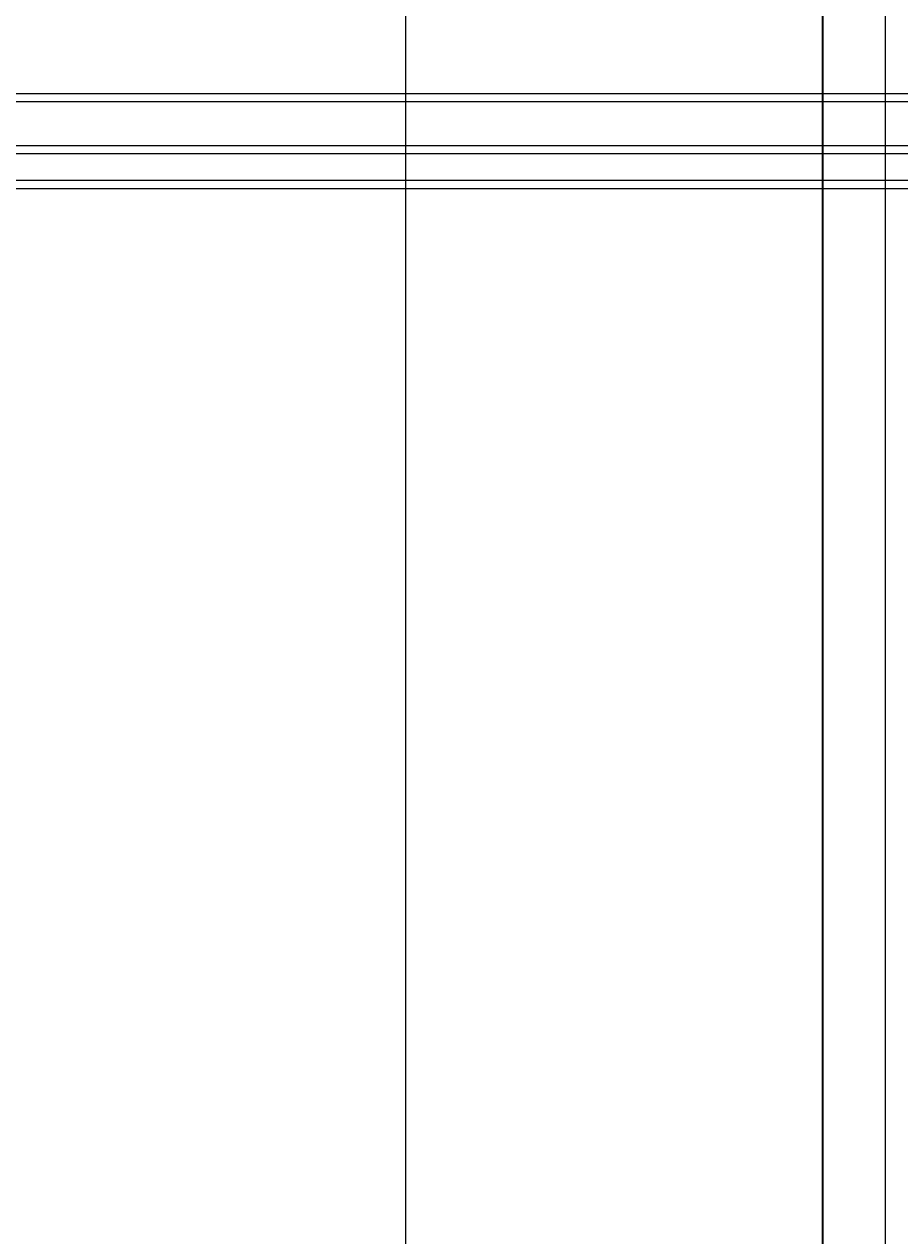
# Model space of a CAD drawing. Units: inches. Extents: x -6 to 289, y -8 to 323.
# Tile 75 of 107: x 248 to 273, y 194 to 229. Entities that reach past the tile are written whole.
import ezdxf

# ---------------------------------------------------------------- set-up
doc = ezdxf.new("R2010")
doc.units = ezdxf.units.IN
doc.header["$MEASUREMENT"] = 0
doc.layers.add('A-ANNO-DIMS', color=2, linetype='Continuous', lineweight=18)
doc.layers.add('A-ELEV', color=7, linetype='Continuous', lineweight=35)
doc.styles.get("Standard").update_dxf_attribs({"font": 'arial.ttf'})
doc.dimstyles.get("Standard").update_dxf_attribs({"dimtxt": 0.18, "dimasz": 0.18, "dimexe": 0.18, "dimexo": 0.0625, "dimgap": 0.09, "dimtad": 0, "dimtih": 1, "dimtoh": 1, "dimdec": 4, "dimzin": 0, "dimdsep": 46, "dimtxsty": 'Standard', "dimcen": 0.09, "dimadec": 0, "dimazin": 0, "dimtfac": 1, "dimtdec": 4, "dimtofl": 0, "dimtmove": 0, "dimatfit": 3, "dimfxl": 1, "dimtolj": 1, "dimtzin": 0, "dimarcsym": 0})

# ---------------------------------------------------------------- blocks, each defined once
blk = doc.blocks.new('*D15')
at = {"layer": 'A-ANNO-DIMS', "color": 0, "lineweight": -2, "transparency": 16777216}
for p, q in [((247.164, 162.411), (247.164, 322.969)), ((271.164, 7.351), (271.164, 322.969)), ((247.344, 322.789), (258.944, 322.789)), ((270.984, 322.789), (259.384, 322.789))]:
    blk.add_line(p, q, dxfattribs=at)
at = {"layer": 'A-ANNO-DIMS', "color": 0, "transparency": 16777216}
for points in [[(247.344, 322.819), (247.344, 322.759), (247.164, 322.789)], [(270.984, 322.819), (270.984, 322.759), (271.164, 322.789)]]:
    blk.add_solid(points, dxfattribs=at)
at = {"layer": 'Defpoints', "color": 0, "transparency": 16777216}
for p in [(271.164, 322.789), (247.164, 162.348), (271.164, 7.289)]:
    blk.add_point(p, dxfattribs=at)
at = {"layer": 'A-ANNO-DIMS', "color": 0, "transparency": 16777216, "insert": (259.164, 322.789), "char_height": 0.18, "attachment_point": 5}
blk.add_mtext('\\A1;24', dxfattribs=at)
blk = doc.blocks.new('*D25')
at = {"layer": 'A-ANNO-DIMS', "color": 0, "lineweight": -2, "transparency": 16777216}
for p, q in [((126.946, 226.654), (288.653, 226.654)), ((288.473, 226.474), (288.473, 202.836)), ((288.473, 178.834), (288.473, 202.472)), ((126.946, 178.654), (288.653, 178.654))]:
    blk.add_line(p, q, dxfattribs=at)
at = {"layer": 'A-ANNO-DIMS', "color": 0, "transparency": 16777216}
for points in [[(288.443, 226.474), (288.503, 226.474), (288.473, 226.654)], [(288.443, 178.834), (288.503, 178.834), (288.473, 178.654)]]:
    blk.add_solid(points, dxfattribs=at)
at = {"layer": 'Defpoints', "color": 0, "transparency": 16777216}
for p in [(126.883, 226.654), (288.473, 226.654), (126.883, 178.654)]:
    blk.add_point(p, dxfattribs=at)
at = {"layer": 'A-ANNO-DIMS', "color": 0, "transparency": 16777216, "insert": (288.473, 202.654), "char_height": 0.18, "attachment_point": 5}
blk.add_mtext('\\A1;48', dxfattribs=at)
blk = doc.blocks.new('*D26')
at = {"layer": 'A-ANNO-DIMS', "color": 0, "lineweight": -2, "transparency": 16777216}
for p, q in [((247.226, 247.289), (288.653, 247.289)), ((288.473, 247.109), (288.473, 237.153)), ((288.473, 226.834), (288.473, 236.789)), ((126.946, 226.654), (288.653, 226.654))]:
    blk.add_line(p, q, dxfattribs=at)
at = {"layer": 'A-ANNO-DIMS', "color": 0, "transparency": 16777216}
for points in [[(288.443, 247.109), (288.503, 247.109), (288.473, 247.289)], [(288.443, 226.834), (288.503, 226.834), (288.473, 226.654)]]:
    blk.add_solid(points, dxfattribs=at)
at = {"layer": 'Defpoints', "color": 0, "transparency": 16777216}
for p in [(247.164, 247.289), (288.473, 247.289), (126.883, 226.654)]:
    blk.add_point(p, dxfattribs=at)
at = {"layer": 'A-ANNO-DIMS', "color": 0, "transparency": 16777216, "insert": (288.473, 236.971), "char_height": 0.18, "attachment_point": 5}
blk.add_mtext('\\A1;20.635', dxfattribs=at)
blk = doc.blocks.new('*D37')
at = {"layer": 'A-ANNO-DIMS', "color": 0, "lineweight": -2, "transparency": 16777216}
for p, q in [((166.446, 224.154), (288.653, 224.154)), ((288.473, 223.974), (288.473, 202.836)), ((288.473, 181.334), (288.473, 202.472)), ((166.446, 181.154), (288.653, 181.154))]:
    blk.add_line(p, q, dxfattribs=at)
at = {"layer": 'A-ANNO-DIMS', "color": 0, "transparency": 16777216}
for points in [[(288.443, 223.974), (288.503, 223.974), (288.473, 224.154)], [(288.443, 181.334), (288.503, 181.334), (288.473, 181.154)]]:
    blk.add_solid(points, dxfattribs=at)
at = {"layer": 'Defpoints', "color": 0, "transparency": 16777216}
for p in [(166.383, 224.154), (288.473, 224.154), (166.383, 181.154)]:
    blk.add_point(p, dxfattribs=at)
at = {"layer": 'A-ANNO-DIMS', "color": 0, "transparency": 16777216, "insert": (288.473, 202.654), "char_height": 0.18, "attachment_point": 5}
blk.add_mtext('\\A1;43', dxfattribs=at)
blk = doc.blocks.new('*D38')
at = {"layer": 'A-ANNO-DIMS', "color": 0, "lineweight": -2, "transparency": 16777216}
for p, q in [((167.446, 225.154), (288.653, 225.154)), ((288.473, 224.974), (288.473, 224.834)), ((288.473, 224.334), (288.473, 224.474)), ((166.446, 224.154), (288.653, 224.154))]:
    blk.add_line(p, q, dxfattribs=at)
at = {"layer": 'A-ANNO-DIMS', "color": 0, "transparency": 16777216}
for points in [[(288.443, 224.974), (288.503, 224.974), (288.473, 225.154)], [(288.443, 224.334), (288.503, 224.334), (288.473, 224.154)]]:
    blk.add_solid(points, dxfattribs=at)
at = {"layer": 'Defpoints', "color": 0, "transparency": 16777216}
for p in [(167.383, 225.154), (288.473, 225.154), (166.383, 224.154)]:
    blk.add_point(p, dxfattribs=at)
at = {"layer": 'A-ANNO-DIMS', "color": 0, "transparency": 16777216, "insert": (288.473, 224.654), "char_height": 0.18, "attachment_point": 5}
blk.add_mtext('\\A1;1', dxfattribs=at)
blk = doc.blocks.new('*D39')
at = {"layer": 'A-ANNO-DIMS', "color": 0, "lineweight": -2, "transparency": 16777216}
for p, q in [((168.946, 226.654), (288.653, 226.654)), ((288.473, 226.474), (288.473, 226.086)), ((288.473, 225.334), (288.473, 225.722)), ((167.446, 225.154), (288.653, 225.154))]:
    blk.add_line(p, q, dxfattribs=at)
at = {"layer": 'A-ANNO-DIMS', "color": 0, "transparency": 16777216}
for points in [[(288.443, 226.474), (288.503, 226.474), (288.473, 226.654)], [(288.443, 225.334), (288.503, 225.334), (288.473, 225.154)]]:
    blk.add_solid(points, dxfattribs=at)
at = {"layer": 'Defpoints', "color": 0, "transparency": 16777216}
for p in [(168.883, 226.654), (288.473, 226.654), (167.383, 225.154)]:
    blk.add_point(p, dxfattribs=at)
at = {"layer": 'A-ANNO-DIMS', "color": 0, "transparency": 16777216, "insert": (288.473, 225.904), "char_height": 0.18, "attachment_point": 5}
blk.add_mtext('\\A1;1.5', dxfattribs=at)
blk = doc.blocks.new('*D47')
at = {"layer": 'A-ANNO-DIMS', "color": 0, "lineweight": -2, "transparency": 16777216}
for p, q in [((233.854, 224.389), (288.653, 224.389)), ((288.473, 224.209), (288.473, 193.55)), ((288.473, 162.528), (288.473, 193.187)), ((236.354, 162.348), (288.653, 162.348))]:
    blk.add_line(p, q, dxfattribs=at)
at = {"layer": 'A-ANNO-DIMS', "color": 0, "transparency": 16777216}
for points in [[(288.443, 224.209), (288.503, 224.209), (288.473, 224.389)], [(288.443, 162.528), (288.503, 162.528), (288.473, 162.348)]]:
    blk.add_solid(points, dxfattribs=at)
at = {"layer": 'Defpoints', "color": 0, "transparency": 16777216}
for p in [(233.792, 224.389), (288.473, 224.389), (236.292, 162.348)]:
    blk.add_point(p, dxfattribs=at)
at = {"layer": 'A-ANNO-DIMS', "color": 0, "transparency": 16777216, "insert": (288.473, 193.369), "char_height": 0.18, "attachment_point": 5}
blk.add_mtext('\\A1;62.04', dxfattribs=at)
blk = doc.blocks.new('*D48')
at = {"layer": 'A-ANNO-DIMS', "color": 0, "lineweight": -2, "transparency": 16777216}
for p, q in [((234.854, 225.389), (288.653, 225.389)), ((288.473, 225.209), (288.473, 225.069)), ((288.473, 224.569), (288.473, 224.708)), ((233.854, 224.389), (288.653, 224.389))]:
    blk.add_line(p, q, dxfattribs=at)
at = {"layer": 'A-ANNO-DIMS', "color": 0, "transparency": 16777216}
for points in [[(288.443, 225.209), (288.503, 225.209), (288.473, 225.389)], [(288.443, 224.569), (288.503, 224.569), (288.473, 224.389)]]:
    blk.add_solid(points, dxfattribs=at)
at = {"layer": 'Defpoints', "color": 0, "transparency": 16777216}
for p in [(234.792, 225.389), (288.473, 225.389), (233.792, 224.389)]:
    blk.add_point(p, dxfattribs=at)
at = {"layer": 'A-ANNO-DIMS', "color": 0, "transparency": 16777216, "insert": (288.473, 224.889), "char_height": 0.18, "attachment_point": 5}
blk.add_mtext('\\A1;1', dxfattribs=at)
blk = doc.blocks.new('*D49')
at = {"layer": 'A-ANNO-DIMS', "color": 0, "lineweight": -2, "transparency": 16777216}
for p, q in [((236.354, 226.889), (288.653, 226.889)), ((288.473, 226.709), (288.473, 226.321)), ((288.473, 225.569), (288.473, 225.957)), ((234.854, 225.389), (288.653, 225.389))]:
    blk.add_line(p, q, dxfattribs=at)
at = {"layer": 'A-ANNO-DIMS', "color": 0, "transparency": 16777216}
for points in [[(288.443, 226.709), (288.503, 226.709), (288.473, 226.889)], [(288.443, 225.569), (288.503, 225.569), (288.473, 225.389)]]:
    blk.add_solid(points, dxfattribs=at)
at = {"layer": 'Defpoints', "color": 0, "transparency": 16777216}
for p in [(236.292, 226.889), (288.473, 226.889), (234.792, 225.389)]:
    blk.add_point(p, dxfattribs=at)
at = {"layer": 'A-ANNO-DIMS', "color": 0, "transparency": 16777216, "insert": (288.473, 226.139), "char_height": 0.18, "attachment_point": 5}
blk.add_mtext('\\A1;1.5', dxfattribs=at)
blk = doc.blocks.new('*D82')
at = {"layer": 'A-ANNO-DIMS', "color": 0, "lineweight": -2, "transparency": 16777216}
for p, q in [((245.215, 66.286), (245.215, 322.969)), ((272.973, 66.286), (272.973, 322.969)), ((245.395, 322.789), (258.699, 322.789)), ((272.793, 322.789), (259.489, 322.789))]:
    blk.add_line(p, q, dxfattribs=at)
at = {"layer": 'A-ANNO-DIMS', "color": 0, "transparency": 16777216}
for points in [[(245.395, 322.819), (245.395, 322.759), (245.215, 322.789)], [(272.793, 322.819), (272.793, 322.759), (272.973, 322.789)]]:
    blk.add_solid(points, dxfattribs=at)
at = {"layer": 'Defpoints', "color": 0, "transparency": 16777216}
for p in [(272.973, 322.789), (245.215, 66.224), (272.973, 66.224)]:
    blk.add_point(p, dxfattribs=at)
at = {"layer": 'A-ANNO-DIMS', "color": 0, "transparency": 16777216, "insert": (259.094, 322.789), "char_height": 0.18, "attachment_point": 5}
blk.add_mtext('\\A1;27.76', dxfattribs=at)
blk = doc.blocks.new('*D100')
at = {"layer": 'A-ANNO-DIMS', "color": 0, "lineweight": -2, "transparency": 16777216}
for p, q in [((247.164, 162.411), (247.164, 322.969)), ((259.164, 139.351), (259.164, 322.969)), ((247.344, 322.789), (252.954, 322.789)), ((258.984, 322.789), (253.373, 322.789))]:
    blk.add_line(p, q, dxfattribs=at)
at = {"layer": 'A-ANNO-DIMS', "color": 0, "transparency": 16777216}
for points in [[(247.344, 322.819), (247.344, 322.759), (247.164, 322.789)], [(258.984, 322.819), (258.984, 322.759), (259.164, 322.789)]]:
    blk.add_solid(points, dxfattribs=at)
at = {"layer": 'Defpoints', "color": 0, "transparency": 16777216}
for p in [(259.164, 322.789), (247.164, 162.348), (259.164, 139.289)]:
    blk.add_point(p, dxfattribs=at)
at = {"layer": 'A-ANNO-DIMS', "color": 0, "transparency": 16777216, "insert": (253.164, 322.789), "char_height": 0.18, "attachment_point": 5}
blk.add_mtext('\\A1;12', dxfattribs=at)

msp = doc.modelspace()

# ---------------------------------------------------------------- linework, layer by layer
at = {"layer": 'A-ELEV'}
msp.add_line((271.1638, 68.4323), (271.1638, 259.2888), dxfattribs=at)

# ---------------------------------------------------------------- dimensions: what is measured, and where the dimension line sits
at = {"layer": 'A-ANNO-DIMS'}
for base, p1, p2, override, picture, middle in [((272.9733, 322.7888), (245.2146, 66.2238), (272.9733, 66.2238), {"dimdec": 2, "dimlfac": 1, "dimrnd": 0, "dimzin": 0, "dimdsep": 46, "dimlunit": 2}, '*D82', (259.0939, 322.7888)), ((271.1638, 322.7888), (247.1638, 162.3484), (271.1638, 7.2888), {"dimdec": 0, "dimlfac": 1, "dimrnd": 0, "dimzin": 0, "dimdsep": 46, "dimlunit": 2}, '*D15', (259.1638, 322.7888)), ((259.1638, 322.7888), (247.1638, 162.3484), (259.1638, 139.2888), {"dimdec": 0, "dimlfac": 1, "dimrnd": 0, "dimzin": 0, "dimdsep": 46, "dimlunit": 2}, '*D100', (253.1638, 322.7888))]:
    dim = msp.add_linear_dim(base=base, p1=p1, p2=p2, dimstyle='Standard', override=override, dxfattribs=at)
    dim.commit()
    dim.dimension.update_dxf_attribs({"geometry": picture, "text_midpoint": middle})
for base, p1, p2, override, picture, middle in [((288.4733, 247.2888), (126.8835, 226.654), (247.1638, 247.2888), {"dimdec": 3, "dimlfac": 1, "dimrnd": 0, "dimzin": 0, "dimdsep": 46, "dimlunit": 2}, '*D26', (288.4733, 236.9714)), ((288.4733, 226.654), (126.8835, 178.654), (126.8835, 226.654), {"dimdec": 0, "dimlfac": 1, "dimrnd": 0, "dimzin": 0, "dimdsep": 46, "dimlunit": 2}, '*D25', (288.4733, 202.654)), ((288.4733, 226.654), (167.3835, 225.154), (168.8835, 226.654), {"dimdec": 1, "dimlfac": 1, "dimrnd": 0, "dimzin": 0, "dimdsep": 46, "dimlunit": 2}, '*D39', (288.4733, 225.904)), ((288.4733, 226.8887), (234.7918, 225.3887), (236.2918, 226.8887), {"dimdec": 1, "dimlfac": 1, "dimrnd": 0, "dimzin": 0, "dimdsep": 46, "dimlunit": 2}, '*D49', (288.4733, 226.1387)), ((288.4733, 225.3887), (233.7918, 224.3887), (234.7918, 225.3887), {"dimdec": 0, "dimlfac": 1, "dimrnd": 0, "dimzin": 0, "dimdsep": 46, "dimlunit": 2}, '*D48', (288.4733, 224.8887)), ((288.4733, 225.154), (166.3835, 224.154), (167.3835, 225.154), {"dimdec": 0, "dimlfac": 1, "dimrnd": 0, "dimzin": 0, "dimdsep": 46, "dimlunit": 2}, '*D38', (288.4733, 224.654)), ((288.4733, 224.3887), (236.2918, 162.3484), (233.7918, 224.3887), {"dimdec": 2, "dimlfac": 1, "dimrnd": 0, "dimzin": 0, "dimdsep": 46, "dimlunit": 2}, '*D47', (288.4733, 193.3685)), ((288.4733, 224.154), (166.3835, 181.154), (166.3835, 224.154), {"dimdec": 0, "dimlfac": 1, "dimrnd": 0, "dimzin": 0, "dimdsep": 46, "dimlunit": 2}, '*D37', (288.4733, 202.654))]:
    dim = msp.add_linear_dim(base=base, p1=p1, p2=p2, angle=90, dimstyle='Standard', override=override, dxfattribs=at)
    dim.commit()
    dim.dimension.update_dxf_attribs({"geometry": picture, "text_midpoint": middle})

doc.saveas('drawing.dxf')
